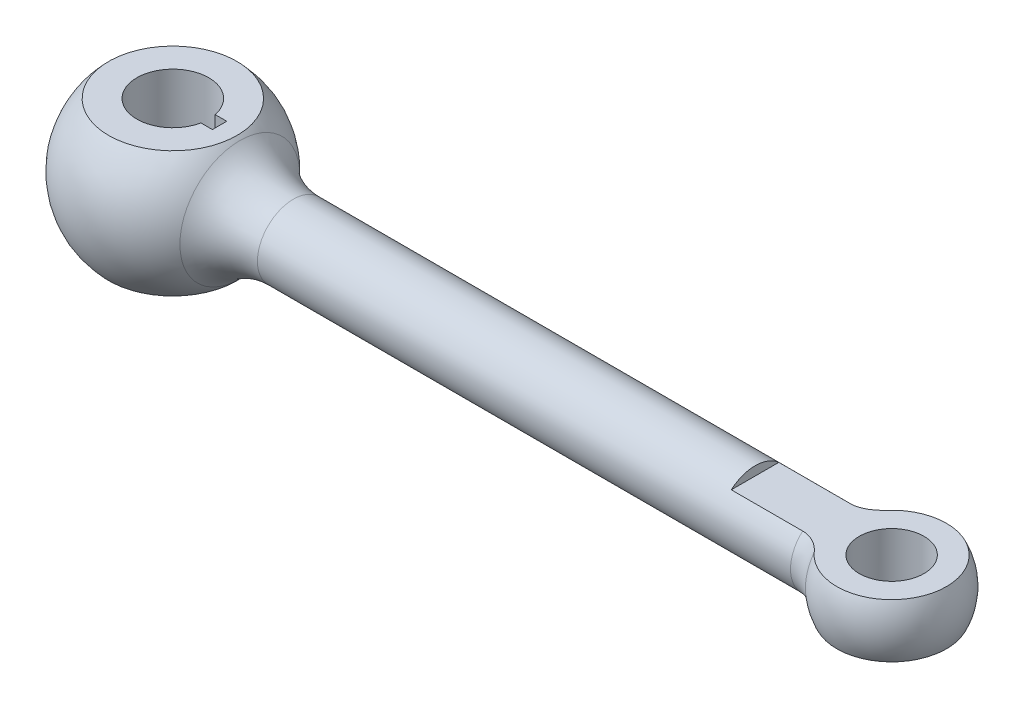
ISO-10303-21;
HEADER;
FILE_DESCRIPTION(('STEP AP214'),'2;1');
FILE_NAME('part.step','',(''),(''),'','','');
FILE_SCHEMA(('AUTOMOTIVE_DESIGN { 1 0 10303 214 1 1 1 1 }'));
ENDSEC;
DATA;
#1=APPLICATION_CONTEXT('core data for automotive mechanical design processes');
#2=APPLICATION_PROTOCOL_DEFINITION('international standard','automotive_design',2000,#1);
#3=PRODUCT_CONTEXT('',#1,'mechanical');
#4=PRODUCT('Part','Part','',(#3));
#5=PRODUCT_RELATED_PRODUCT_CATEGORY('part','',(#4));
#6=PRODUCT_DEFINITION_FORMATION('','',#4);
#7=PRODUCT_DEFINITION_CONTEXT('part definition',#1,'design');
#8=PRODUCT_DEFINITION('design','',#6,#7);
#9=PRODUCT_DEFINITION_SHAPE('','',#8);
#10=(LENGTH_UNIT() NAMED_UNIT(*) SI_UNIT(.MILLI.,.METRE.));
#11=(NAMED_UNIT(*) PLANE_ANGLE_UNIT() SI_UNIT($,.RADIAN.));
#12=(NAMED_UNIT(*) SI_UNIT($,.STERADIAN.) SOLID_ANGLE_UNIT());
#13=UNCERTAINTY_MEASURE_WITH_UNIT(LENGTH_MEASURE(1.E-05),#10,'distance_accuracy_value','');
#14=(GEOMETRIC_REPRESENTATION_CONTEXT(3) GLOBAL_UNCERTAINTY_ASSIGNED_CONTEXT((#13)) GLOBAL_UNIT_ASSIGNED_CONTEXT((#10,
#11,#12)) REPRESENTATION_CONTEXT('',''));
#15=CARTESIAN_POINT('',(0.,0.,0.));
#16=DIRECTION('',(0.,0.,1.));
#17=DIRECTION('',(1.,0.,0.));
#18=AXIS2_PLACEMENT_3D('',#15,#16,#17);
#19=CARTESIAN_POINT('',(-25.,0.,0.));
#20=DIRECTION('',(-1.,0.,0.));
#21=DIRECTION('',(0.,1.,0.));
#22=AXIS2_PLACEMENT_3D('',#19,#20,#21);
#23=SPHERICAL_SURFACE('',#22,25.);
#24=CARTESIAN_POINT('',(-6.36610018750175,0.,0.));
#25=DIRECTION('',(-1.,0.,0.));
#26=DIRECTION('',(0.,0.,1.));
#27=AXIS2_PLACEMENT_3D('',#24,#25,#26);
#28=CIRCLE('',#27,16.6666666666667);
#29=CARTESIAN_POINT('',(-6.36610018750175,0.,16.6666666666667));
#30=VERTEX_POINT('',#29);
#31=EDGE_CURVE('E198',#30,#30,#28,.T.);
#32=ORIENTED_EDGE('',*,*,#31,.T.);
#33=EDGE_LOOP('',(#32));
#34=FACE_BOUND('',#33,.T.);
#35=CARTESIAN_POINT('',(-25.,17.5,0.));
#36=DIRECTION('',(0.,1.,0.));
#37=DIRECTION('',(0.,0.,1.));
#38=AXIS2_PLACEMENT_3D('',#35,#36,#37);
#39=CIRCLE('',#38,17.8535710713571);
#40=CARTESIAN_POINT('',(-25.,17.5,17.8535710713571));
#41=VERTEX_POINT('',#40);
#42=EDGE_CURVE('E164',#41,#41,#39,.T.);
#43=ORIENTED_EDGE('',*,*,#42,.F.);
#44=EDGE_LOOP('',(#43));
#45=FACE_BOUND('',#44,.T.);
#46=CARTESIAN_POINT('',(-25.,-17.5,0.));
#47=DIRECTION('',(0.,-1.,0.));
#48=DIRECTION('',(0.,0.,-1.));
#49=AXIS2_PLACEMENT_3D('',#46,#47,#48);
#50=CIRCLE('',#49,17.8535710713571);
#51=CARTESIAN_POINT('',(-25.,-17.5,-17.8535710713571));
#52=VERTEX_POINT('',#51);
#53=EDGE_CURVE('E156',#52,#52,#50,.T.);
#54=ORIENTED_EDGE('',*,*,#53,.F.);
#55=EDGE_LOOP('',(#54));
#56=FACE_BOUND('',#55,.T.);
#57=CARTESIAN_POINT('',(-49.6779253585061,0.,0.));
#58=DIRECTION('',(1.,0.,0.));
#59=DIRECTION('',(0.,0.,-1.));
#60=AXIS2_PLACEMENT_3D('',#57,#58,#59);
#61=CIRCLE('',#60,4.);
#62=CARTESIAN_POINT('',(-49.6779253585061,0.,-4.));
#63=VERTEX_POINT('',#62);
#64=EDGE_CURVE('E293',#63,#63,#61,.F.);
#65=ORIENTED_EDGE('',*,*,#64,.F.);
#66=EDGE_LOOP('',(#65));
#67=FACE_BOUND('',#66,.T.);
#68=ADVANCED_FACE('F41',(#34,#45,#56,#67),#23,.T.);
#69=CARTESIAN_POINT('',(-25.,-22.5,0.));
#70=DIRECTION('',(0.,1.,0.));
#71=DIRECTION('',(0.,0.,1.));
#72=AXIS2_PLACEMENT_3D('',#69,#70,#71);
#73=CYLINDRICAL_SURFACE('',#72,10.);
#74=CARTESIAN_POINT('',(-25.,-17.5,0.));
#75=DIRECTION('',(0.,-1.,0.));
#76=DIRECTION('',(0.,0.,-1.));
#77=AXIS2_PLACEMENT_3D('',#74,#75,#76);
#78=CIRCLE('',#77,10.);
#79=CARTESIAN_POINT('',(-15.2020410288673,-17.5,2.));
#80=VERTEX_POINT('',#79);
#81=CARTESIAN_POINT('',(-15.2020410288673,-17.5,-2.));
#82=VERTEX_POINT('',#81);
#83=EDGE_CURVE('E133',#80,#82,#78,.T.);
#84=ORIENTED_EDGE('',*,*,#83,.T.);
#85=DIRECTION('',(0.,1.,0.));
#86=VECTOR('',#85,1.);
#87=CARTESIAN_POINT('',(-15.2020410288673,-22.5,-2.));
#88=LINE('',#87,#86);
#89=CARTESIAN_POINT('',(-15.2020410288673,17.5,-2.));
#90=VERTEX_POINT('',#89);
#91=EDGE_CURVE('E121',#82,#90,#88,.T.);
#92=ORIENTED_EDGE('',*,*,#91,.T.);
#93=CARTESIAN_POINT('',(-25.,17.5,0.));
#94=DIRECTION('',(0.,1.,0.));
#95=DIRECTION('',(0.,0.,1.));
#96=AXIS2_PLACEMENT_3D('',#93,#94,#95);
#97=CIRCLE('',#96,10.);
#98=CARTESIAN_POINT('',(-15.2020410288673,17.5,2.));
#99=VERTEX_POINT('',#98);
#100=EDGE_CURVE('E129',#90,#99,#97,.T.);
#101=ORIENTED_EDGE('',*,*,#100,.T.);
#102=DIRECTION('',(0.,1.,0.));
#103=VECTOR('',#102,1.);
#104=CARTESIAN_POINT('',(-15.2020410288673,-22.5,2.));
#105=LINE('',#104,#103);
#106=EDGE_CURVE('E138',#80,#99,#105,.T.);
#107=ORIENTED_EDGE('',*,*,#106,.F.);
#108=EDGE_LOOP('',(#84,#92,#101,#107));
#109=FACE_BOUND('',#108,.T.);
#110=CARTESIAN_POINT('',(-34.1651513899117,0.,4.));
#111=CARTESIAN_POINT('',(-34.1651522072251,-0.107177496784384,3.99999917996685));
#112=CARTESIAN_POINT('',(-34.1670378270459,-0.214387859794794,3.99568627578832));
#113=CARTESIAN_POINT('',(-34.1745189058127,-0.428032094170665,3.97847804504315));
#114=CARTESIAN_POINT('',(-34.1801166353845,-0.534465449945316,3.965577465543));
#115=CARTESIAN_POINT('',(-34.1948507861607,-0.745935953355521,3.9312935770878));
#116=CARTESIAN_POINT('',(-34.2039942584833,-0.850969884848686,3.90989336356571));
#117=CARTESIAN_POINT('',(-34.2255144619826,-1.05868759718977,3.85883937208579));
#118=CARTESIAN_POINT('',(-34.2378925354171,-1.16137038310176,3.82918216740128));
#119=CARTESIAN_POINT('',(-34.2792023148764,-1.46398972662859,3.72849978450445));
#120=CARTESIAN_POINT('',(-34.3123881019352,-1.65953792096433,3.64559228099563));
#121=CARTESIAN_POINT('',(-34.3862951267144,-2.03380126867295,3.45083256453889));
#122=CARTESIAN_POINT('',(-34.4270147185353,-2.21252008589124,3.33898667159604));
#123=CARTESIAN_POINT('',(-34.5140167746093,-2.55851181360141,3.08264624953204));
#124=CARTESIAN_POINT('',(-34.5604782179202,-2.72471043328898,2.93675933272146));
#125=CARTESIAN_POINT('',(-34.6522492808802,-3.03106040804192,2.61941759406606));
#126=CARTESIAN_POINT('',(-34.6975584932633,-3.17120266075496,2.44795387495429));
#127=CARTESIAN_POINT('',(-34.7840681180817,-3.42681210983709,2.07601279575004));
#128=CARTESIAN_POINT('',(-34.8250360629585,-3.54108841996941,1.87465797803874));
#129=CARTESIAN_POINT('',(-34.8960785633395,-3.73368731967694,1.45365059895514));
#130=CARTESIAN_POINT('',(-34.9261575504962,-3.81202453943324,1.23400552632834));
#131=CARTESIAN_POINT('',(-34.9707664974986,-3.92668292732297,0.793932865332428));
#132=CARTESIAN_POINT('',(-34.9859787347939,-3.96485461599806,0.574057972725524));
#133=CARTESIAN_POINT('',(-35.001606214367,-4.00405698350082,0.130532654160158));
#134=CARTESIAN_POINT('',(-35.0020269755724,-4.0051015150445,-0.0931163324631207));
#135=CARTESIAN_POINT('',(-34.9884392562601,-3.97103445745354,-0.524464988663932));
#136=CARTESIAN_POINT('',(-34.9752399353889,-3.93795045370289,-0.732354905542457));
#137=CARTESIAN_POINT('',(-34.9369858294236,-3.8400142481818,-1.1393462186423));
#138=CARTESIAN_POINT('',(-34.9119301744378,-3.77515971541564,-1.33844696883603));
#139=CARTESIAN_POINT('',(-34.8519364891382,-3.61472703402771,-1.72579587696675));
#140=CARTESIAN_POINT('',(-34.8168552093215,-3.51870057031128,-1.91383524674319));
#141=CARTESIAN_POINT('',(-34.7402917036085,-3.29906998621966,-2.27161630149723));
#142=CARTESIAN_POINT('',(-34.6988072853438,-3.17545641381566,-2.44135168543995));
#143=CARTESIAN_POINT('',(-34.6104327435216,-2.8947017280952,-2.76953765597606));
#144=CARTESIAN_POINT('',(-34.5633665302349,-2.73589221484983,-2.92651569053149));
#145=CARTESIAN_POINT('',(-34.4712332194655,-2.39401885634057,-3.21221483078645));
#146=CARTESIAN_POINT('',(-34.4261667801616,-2.21094710361003,-3.34092668757428));
#147=CARTESIAN_POINT('',(-34.3419379481804,-1.81916195525085,-3.56980837743822));
#148=CARTESIAN_POINT('',(-34.3029782811541,-1.60987033932236,-3.66906930327244));
#149=CARTESIAN_POINT('',(-34.2377518068817,-1.1755690193759,-3.83035251973301));
#150=CARTESIAN_POINT('',(-34.2114767578262,-0.950569630546911,-3.89239899675599));
#151=CARTESIAN_POINT('',(-34.1765951940543,-0.50592844506505,-3.97390989770977));
#152=CARTESIAN_POINT('',(-34.1670073291228,-0.286799105742873,-3.99574419362908));
#153=CARTESIAN_POINT('',(-34.1637899573808,0.152154415519103,-4.00312265288578));
#154=CARTESIAN_POINT('',(-34.1701556112072,0.371978366551337,-3.98867782118257));
#155=CARTESIAN_POINT('',(-34.1971208871823,0.792917869913856,-3.92606578958006));
#156=CARTESIAN_POINT('',(-34.216889155966,0.994385874799997,-3.87986612404771));
#157=CARTESIAN_POINT('',(-34.2674010205468,1.38657680957103,-3.75760837382175));
#158=CARTESIAN_POINT('',(-34.2981470497719,1.57729734621477,-3.68154366860459));
#159=CARTESIAN_POINT('',(-34.368675637202,1.95120471559083,-3.49827127896311));
#160=CARTESIAN_POINT('',(-34.4087740927836,2.13377237738722,-3.38992573652914));
#161=CARTESIAN_POINT('',(-34.4930077031559,2.47896597488502,-3.14633044888379));
#162=CARTESIAN_POINT('',(-34.5371444979208,2.64158374559781,-3.01106974696435));
#163=CARTESIAN_POINT('',(-34.6284183194284,2.95474681719132,-2.70568842336055));
#164=CARTESIAN_POINT('',(-34.6755361457051,3.10351313055453,-2.53373085888854));
#165=CARTESIAN_POINT('',(-34.7643958913502,3.3703541532482,-2.16616726673934));
#166=CARTESIAN_POINT('',(-34.8061375918612,3.48842761329747,-1.97056027694192));
#167=CARTESIAN_POINT('',(-34.8796743180093,3.69009525281948,-1.56055986799732));
#168=CARTESIAN_POINT('',(-34.9114717248188,3.77369768794723,-1.346170961965));
#169=CARTESIAN_POINT('',(-34.9614542693725,3.90309770519939,-0.904787181861568));
#170=CARTESIAN_POINT('',(-34.9796467941012,3.94891580431339,-0.677799220674799));
#171=CARTESIAN_POINT('',(-34.9995801642567,3.99900940191103,-0.233633020611975));
#172=CARTESIAN_POINT('',(-35.0023169350655,4.00580025207679,-0.0167809848943052));
#173=CARTESIAN_POINT('',(-34.9937208474038,3.98428904627956,0.414867671174724));
#174=CARTESIAN_POINT('',(-34.9823901187126,3.95599230247905,0.62966459770289));
#175=CARTESIAN_POINT('',(-34.9474302678916,3.86690640578721,1.04434180494581));
#176=CARTESIAN_POINT('',(-34.9241896149174,3.80714204349495,1.2444776131699));
#177=CARTESIAN_POINT('',(-34.8678989544096,3.65789445524216,1.63184470564404));
#178=CARTESIAN_POINT('',(-34.8348471377614,3.56840574794402,1.81907360209111));
#179=CARTESIAN_POINT('',(-34.7603618958876,3.3577933524316,2.18440609879393));
#180=CARTESIAN_POINT('',(-34.7186226276455,3.23544645590386,2.3617408310488));
#181=CARTESIAN_POINT('',(-34.6317880306343,2.96442391636386,2.69410799958837));
#182=CARTESIAN_POINT('',(-34.5866913172977,2.81573737596091,2.84913115669899));
#183=CARTESIAN_POINT('',(-34.4947554025592,2.48536576113423,3.14240275826141));
#184=CARTESIAN_POINT('',(-34.4479811565371,2.30220770129796,3.27901865020172));
#185=CARTESIAN_POINT('',(-34.3609929250149,1.91413027875233,3.51969402497221));
#186=CARTESIAN_POINT('',(-34.3207797110774,1.70920836133381,3.62374968011082));
#187=CARTESIAN_POINT('',(-34.2551790064237,1.30187605622044,3.78798515690828));
#188=CARTESIAN_POINT('',(-34.228784514946,1.10089232405414,3.85126569346865));
#189=CARTESIAN_POINT('',(-34.1988556584339,0.793361040209279,3.92194632104984));
#190=CARTESIAN_POINT('',(-34.1904927063377,0.68992696410562,3.94146052144918));
#191=CARTESIAN_POINT('',(-34.1772120034161,0.481643070389122,3.97228850679684));
#192=CARTESIAN_POINT('',(-34.1722922529317,0.376794110604086,3.98360705155155));
#193=CARTESIAN_POINT('',(-34.1678367542342,0.226449408647594,3.99384232103283));
#194=CARTESIAN_POINT('',(-34.1668305981541,0.181200169677813,3.99615058414993));
#195=CARTESIAN_POINT('',(-34.1654877186478,0.0906359157853919,3.99922965337524));
#196=CARTESIAN_POINT('',(-34.1651510443039,0.0453208962838169,4.00000034675784));
#197=CARTESIAN_POINT('',(-34.1651513899117,0.,4.));
#198=B_SPLINE_CURVE_WITH_KNOTS('',3,(#110,#111,#112,#113,#114,#115,#116,#117,#118,#119,#120,
#121,#122,#123,#124,#125,#126,#127,#128,#129,#130,#131,#132,#133,#134,#135,#136,#137,#138,#139,
#140,#141,#142,#143,#144,#145,#146,#147,#148,#149,#150,#151,#152,#153,#154,#155,#156,#157,#158,
#159,#160,#161,#162,#163,#164,#165,#166,#167,#168,#169,#170,#171,#172,#173,#174,#175,#176,#177,
#178,#179,#180,#181,#182,#183,#184,#185,#186,#187,#188,#189,#190,#191,#192,#193,#194,#195,#196,
#197),.UNSPECIFIED.,.T.,.F.,(4,2,2,2,2,2,2,2,2,2,2,2,2,2,2,2,2,2,2,2,2,2,2,2,2,2,2,2,2,2,2,2,2,
2,2,2,2,2,2,2,2,2,2,4),(0.,0.321486083338404,0.64316899511119,0.965494918272705,
1.28795480954363,1.92974178448592,2.57138871437637,3.24631250358764,3.92147162486599,
4.62325351972771,5.32474947728875,5.99228379564281,6.65956904401258,7.28937303450519,
7.91922324048033,8.5585661425971,9.19812843669976,9.87968101952625,10.5614562804417,
11.2624893122443,11.9630662339012,12.6208430883876,13.2784204360579,13.898545099602,
14.5188073109319,15.1642232309532,15.8099024284161,16.5032748228387,17.1966754349541,
17.8899098841554,18.5827676569819,19.2304209330182,19.8779761681512,20.5056400267662,
21.1334196944708,21.7889411606976,22.4447344691833,23.1411252036114,23.8375977730829,
24.4715333542807,24.7879924179096,25.1042675432749,25.240200643082,25.3761437083411),.UNSPECIFIED.);
#199=CARTESIAN_POINT('',(-34.1651513899117,0.,4.));
#200=VERTEX_POINT('',#199);
#201=EDGE_CURVE('E46',#200,#200,#198,.T.);
#202=ORIENTED_EDGE('',*,*,#201,.F.);
#203=EDGE_LOOP('',(#202));
#204=FACE_BOUND('',#203,.T.);
#205=ADVANCED_FACE('F126',(#109,#204),#73,.F.);
#206=CARTESIAN_POINT('',(175.,0.,0.));
#207=DIRECTION('',(-1.,0.,0.));
#208=DIRECTION('',(0.,1.,0.));
#209=AXIS2_PLACEMENT_3D('',#206,#207,#208);
#210=SPHERICAL_SURFACE('',#209,17.);
#211=CARTESIAN_POINT('',(175.,-7.5,0.));
#212=DIRECTION('',(0.,-1.,0.));
#213=DIRECTION('',(0.,0.,-1.));
#214=AXIS2_PLACEMENT_3D('',#211,#212,#213);
#215=CIRCLE('',#214,15.2561463023924);
#216=CARTESIAN_POINT('',(163.579552907308,-7.5,-10.1155023702739));
#217=VERTEX_POINT('',#216);
#218=CARTESIAN_POINT('',(163.579552907308,-7.5,10.1155023702739));
#219=VERTEX_POINT('',#218);
#220=EDGE_CURVE('E165',#217,#219,#215,.T.);
#221=ORIENTED_EDGE('',*,*,#220,.F.);
#222=CARTESIAN_POINT('',(163.579552907308,0.,0.));
#223=DIRECTION('',(1.,0.,0.));
#224=DIRECTION('',(0.,0.,-1.));
#225=AXIS2_PLACEMENT_3D('',#222,#223,#224);
#226=CIRCLE('',#225,12.5925925925926);
#227=CARTESIAN_POINT('',(163.579552907308,7.5,-10.1155023702739));
#228=VERTEX_POINT('',#227);
#229=EDGE_CURVE('E62',#217,#228,#226,.T.);
#230=ORIENTED_EDGE('',*,*,#229,.T.);
#231=CARTESIAN_POINT('',(175.,7.5,0.));
#232=DIRECTION('',(0.,1.,0.));
#233=DIRECTION('',(0.,0.,1.));
#234=AXIS2_PLACEMENT_3D('',#231,#232,#233);
#235=CIRCLE('',#234,15.2561463023924);
#236=CARTESIAN_POINT('',(163.579552907308,7.5,10.1155023702739));
#237=VERTEX_POINT('',#236);
#238=EDGE_CURVE('E167',#237,#228,#235,.T.);
#239=ORIENTED_EDGE('',*,*,#238,.F.);
#240=CARTESIAN_POINT('',(163.579552907308,0.,0.));
#241=DIRECTION('',(1.,0.,0.));
#242=DIRECTION('',(0.,0.,-1.));
#243=AXIS2_PLACEMENT_3D('',#240,#241,#242);
#244=CIRCLE('',#243,12.5925925925926);
#245=EDGE_CURVE('E213',#237,#219,#244,.T.);
#246=ORIENTED_EDGE('',*,*,#245,.T.);
#247=EDGE_LOOP('',(#221,#230,#239,#246));
#248=FACE_BOUND('',#247,.T.);
#249=ADVANCED_FACE('F262',(#248),#210,.T.);
#250=CARTESIAN_POINT('',(0.,0.,0.));
#251=DIRECTION('',(-1.,0.,0.));
#252=DIRECTION('',(0.,0.,1.));
#253=AXIS2_PLACEMENT_3D('',#250,#251,#252);
#254=CYLINDRICAL_SURFACE('',#253,10.);
#255=CARTESIAN_POINT('',(8.54101966249685,0.,0.));
#256=DIRECTION('',(-1.,0.,0.));
#257=DIRECTION('',(0.,0.,1.));
#258=AXIS2_PLACEMENT_3D('',#255,#256,#257);
#259=CIRCLE('',#258,10.);
#260=CARTESIAN_POINT('',(8.54101966249685,0.,10.));
#261=VERTEX_POINT('',#260);
#262=EDGE_CURVE('E202',#261,#261,#259,.F.);
#263=ORIENTED_EDGE('',*,*,#262,.T.);
#264=EDGE_LOOP('',(#263));
#265=FACE_BOUND('',#264,.T.);
#266=DIRECTION('',(-1.,0.,0.));
#267=VECTOR('',#266,1.);
#268=CARTESIAN_POINT('',(0.,7.5,-6.61437827766147));
#269=LINE('',#268,#267);
#270=CARTESIAN_POINT('',(156.861642852783,7.5,-6.61437827766147));
#271=VERTEX_POINT('',#270);
#272=CARTESIAN_POINT('',(137.002179540985,7.5,-6.61437827766147));
#273=VERTEX_POINT('',#272);
#274=EDGE_CURVE('E180',#271,#273,#269,.T.);
#275=ORIENTED_EDGE('',*,*,#274,.F.);
#276=CARTESIAN_POINT('',(156.861642852783,0.,0.));
#277=DIRECTION('',(1.,0.,0.));
#278=DIRECTION('',(0.,0.,-1.));
#279=AXIS2_PLACEMENT_3D('',#276,#277,#278);
#280=CIRCLE('',#279,10.);
#281=CARTESIAN_POINT('',(156.861642852783,-7.5,-6.61437827766147));
#282=VERTEX_POINT('',#281);
#283=EDGE_CURVE('E211',#271,#282,#280,.F.);
#284=ORIENTED_EDGE('',*,*,#283,.T.);
#285=DIRECTION('',(-1.,0.,0.));
#286=VECTOR('',#285,1.);
#287=CARTESIAN_POINT('',(0.,-7.5,-6.61437827766147));
#288=LINE('',#287,#286);
#289=CARTESIAN_POINT('',(137.002179540985,-7.5,-6.61437827766147));
#290=VERTEX_POINT('',#289);
#291=EDGE_CURVE('E177',#290,#282,#288,.F.);
#292=ORIENTED_EDGE('',*,*,#291,.F.);
#293=CARTESIAN_POINT('',(137.002179540985,0.,0.));
#294=DIRECTION('',(-1.,0.,0.));
#295=DIRECTION('',(0.,0.,1.));
#296=AXIS2_PLACEMENT_3D('',#293,#294,#295);
#297=CIRCLE('',#296,10.);
#298=CARTESIAN_POINT('',(137.002179540985,-7.5,6.61437827766147));
#299=VERTEX_POINT('',#298);
#300=EDGE_CURVE('E185',#290,#299,#297,.T.);
#301=ORIENTED_EDGE('',*,*,#300,.T.);
#302=DIRECTION('',(-1.,0.,0.));
#303=VECTOR('',#302,1.);
#304=CARTESIAN_POINT('',(0.,-7.5,6.61437827766147));
#305=LINE('',#304,#303);
#306=CARTESIAN_POINT('',(156.861642852783,-7.5,6.61437827766147));
#307=VERTEX_POINT('',#306);
#308=EDGE_CURVE('E184',#307,#299,#305,.T.);
#309=ORIENTED_EDGE('',*,*,#308,.F.);
#310=CARTESIAN_POINT('',(156.861642852783,0.,0.));
#311=DIRECTION('',(1.,0.,0.));
#312=DIRECTION('',(0.,0.,-1.));
#313=AXIS2_PLACEMENT_3D('',#310,#311,#312);
#314=CIRCLE('',#313,10.);
#315=CARTESIAN_POINT('',(156.861642852783,7.5,6.61437827766147));
#316=VERTEX_POINT('',#315);
#317=EDGE_CURVE('E206',#307,#316,#314,.F.);
#318=ORIENTED_EDGE('',*,*,#317,.T.);
#319=DIRECTION('',(-1.,0.,0.));
#320=VECTOR('',#319,1.);
#321=CARTESIAN_POINT('',(0.,7.5,6.61437827766147));
#322=LINE('',#321,#320);
#323=CARTESIAN_POINT('',(137.002179540985,7.5,6.61437827766147));
#324=VERTEX_POINT('',#323);
#325=EDGE_CURVE('E175',#324,#316,#322,.F.);
#326=ORIENTED_EDGE('',*,*,#325,.F.);
#327=CARTESIAN_POINT('',(137.002179540985,0.,0.));
#328=DIRECTION('',(1.,0.,0.));
#329=DIRECTION('',(0.,0.,-1.));
#330=AXIS2_PLACEMENT_3D('',#327,#328,#329);
#331=CIRCLE('',#330,10.);
#332=EDGE_CURVE('E172',#273,#324,#331,.T.);
#333=ORIENTED_EDGE('',*,*,#332,.F.);
#334=EDGE_LOOP('',(#275,#284,#292,#301,#309,#318,#326,#333));
#335=FACE_BOUND('',#334,.T.);
#336=ADVANCED_FACE('F259',(#265,#335),#254,.T.);
#337=CARTESIAN_POINT('',(137.002179540985,17.5,-20.2694187702266));
#338=DIRECTION('',(1.,0.,0.));
#339=DIRECTION('',(0.,0.,-1.));
#340=AXIS2_PLACEMENT_3D('',#337,#338,#339);
#341=PLANE('',#340);
#342=ORIENTED_EDGE('',*,*,#332,.T.);
#343=DIRECTION('',(0.,0.,1.));
#344=VECTOR('',#343,1.);
#345=CARTESIAN_POINT('',(137.002179540985,7.5,-20.2694187702266));
#346=LINE('',#345,#344);
#347=EDGE_CURVE('E166',#273,#324,#346,.T.);
#348=ORIENTED_EDGE('',*,*,#347,.F.);
#349=EDGE_LOOP('',(#342,#348));
#350=FACE_BOUND('',#349,.T.);
#351=ADVANCED_FACE('F253',(#350),#341,.T.);
#352=CARTESIAN_POINT('',(0.,7.5,0.));
#353=DIRECTION('',(0.,1.,0.));
#354=DIRECTION('',(0.,0.,1.));
#355=AXIS2_PLACEMENT_3D('',#352,#353,#354);
#356=PLANE('',#355);
#357=CARTESIAN_POINT('',(175.,7.5,0.));
#358=DIRECTION('',(0.,1.,0.));
#359=DIRECTION('',(0.,0.,1.));
#360=AXIS2_PLACEMENT_3D('',#357,#358,#359);
#361=CIRCLE('',#360,9.00000000000001);
#362=CARTESIAN_POINT('',(175.,7.5,9.00000000000001));
#363=VERTEX_POINT('',#362);
#364=EDGE_CURVE('E205',#363,#363,#361,.T.);
#365=ORIENTED_EDGE('',*,*,#364,.F.);
#366=EDGE_LOOP('',(#365));
#367=FACE_BOUND('',#366,.T.);
#368=ORIENTED_EDGE('',*,*,#238,.T.);
#369=CARTESIAN_POINT('',(163.579552907308,7.5,-10.1155023702739));
#370=CARTESIAN_POINT('',(163.474769834163,7.5,-9.99720726138382));
#371=CARTESIAN_POINT('',(163.3678618628,7.5,-9.88080970811956));
#372=CARTESIAN_POINT('',(163.149837656753,7.5,-9.65200955610534));
#373=CARTESIAN_POINT('',(163.038721113773,7.5,-9.53960725119778));
#374=CARTESIAN_POINT('',(162.698727604228,7.5,-9.20831245884123));
#375=CARTESIAN_POINT('',(162.463593029927,7.5,-8.99576936234443));
#376=CARTESIAN_POINT('',(161.973130319847,7.5,-8.58661619341136));
#377=CARTESIAN_POINT('',(161.717532005201,7.5,-8.39032873131534));
#378=CARTESIAN_POINT('',(161.190347543977,7.5,-8.02110441295629));
#379=CARTESIAN_POINT('',(160.918775780457,7.5,-7.84814699808274));
#380=CARTESIAN_POINT('',(160.26295451581,7.5,-7.47440052714146));
#381=CARTESIAN_POINT('',(159.872185695544,7.5,-7.28463335372538));
#382=CARTESIAN_POINT('',(159.269067190411,7.5,-7.04814733941781));
#383=CARTESIAN_POINT('',(159.065931678387,7.5,-6.97750828643357));
#384=CARTESIAN_POINT('',(158.65444068621,7.5,-6.85369940596053));
#385=CARTESIAN_POINT('',(158.446087612678,7.5,-6.80052167847359));
#386=CARTESIAN_POINT('',(158.01048008529,7.5,-6.71025341266789));
#387=CARTESIAN_POINT('',(157.782929072302,7.5,-6.67456227561141));
#388=CARTESIAN_POINT('',(157.439215061707,7.5,-6.63858866966147));
#389=CARTESIAN_POINT('',(157.323917836321,7.5,-6.62952413667485));
#390=CARTESIAN_POINT('',(157.092968815727,7.5,-6.61741406589461));
#391=CARTESIAN_POINT('',(156.977316912966,7.5,-6.61437058275184));
#392=CARTESIAN_POINT('',(156.861642852783,7.5,-6.61437827766147));
#393=B_SPLINE_CURVE_WITH_KNOTS('',3,(#369,#370,#371,#372,#373,#374,#375,#376,#377,#378,#379,
#380,#381,#382,#383,#384,#385,#386,#387,#388,#389,#390,#391,#392),.UNSPECIFIED.,.F.,.F.,(4,2,2,
2,2,2,2,2,2,2,2,4),(0.,0.474036656551859,0.948108105696828,1.89799697678677,2.86363556209121,
3.82841758163828,5.12644490386445,5.77101491101689,6.41529289334001,7.10501836282089,
7.45183935202879,7.79877867163184),.UNSPECIFIED.);
#394=EDGE_CURVE('E224',#228,#271,#393,.T.);
#395=ORIENTED_EDGE('',*,*,#394,.T.);
#396=ORIENTED_EDGE('',*,*,#274,.T.);
#397=ORIENTED_EDGE('',*,*,#347,.T.);
#398=ORIENTED_EDGE('',*,*,#325,.T.);
#399=CARTESIAN_POINT('',(156.861642852783,7.5,6.61437827766147));
#400=CARTESIAN_POINT('',(156.978718981189,7.5,6.61436537547752));
#401=CARTESIAN_POINT('',(157.095790003373,7.5,6.61748635841604));
#402=CARTESIAN_POINT('',(157.329586048896,7.5,6.62989960137549));
#403=CARTESIAN_POINT('',(157.446311125305,7.5,6.63919085972964));
#404=CARTESIAN_POINT('',(157.678890680255,7.5,6.66382417376256));
#405=CARTESIAN_POINT('',(157.794746412737,7.5,6.67915439326618));
#406=CARTESIAN_POINT('',(158.025521155016,7.5,6.71568182750459));
#407=CARTESIAN_POINT('',(158.140440137299,7.5,6.73687921394221));
#408=CARTESIAN_POINT('',(158.480369960769,7.5,6.80831037403592));
#409=CARTESIAN_POINT('',(158.703705459786,7.5,6.86672863148083));
#410=CARTESIAN_POINT('',(159.144207461786,7.5,7.0034637798633));
#411=CARTESIAN_POINT('',(159.361371112734,7.5,7.08178970917642));
#412=CARTESIAN_POINT('',(159.786670880194,7.5,7.25530329193259));
#413=CARTESIAN_POINT('',(159.994867796626,7.5,7.35034279209469));
#414=CARTESIAN_POINT('',(160.403562374738,7.5,7.55562714513321));
#415=CARTESIAN_POINT('',(160.604060514978,7.5,7.66587105093353));
#416=CARTESIAN_POINT('',(160.998074881118,7.5,7.90036091770959));
#417=CARTESIAN_POINT('',(161.191549310851,7.5,8.02467680582048));
#418=CARTESIAN_POINT('',(161.570233804941,7.5,8.28531892470298));
#419=CARTESIAN_POINT('',(161.75544317311,7.5,8.4216461643554));
#420=CARTESIAN_POINT('',(162.085608824903,7.5,8.68013427269151));
#421=CARTESIAN_POINT('',(162.231919209356,7.5,8.8005745126537));
#422=CARTESIAN_POINT('',(162.518724288325,7.5,9.04817416826897));
#423=CARTESIAN_POINT('',(162.659219307179,7.5,9.17533320829355));
#424=CARTESIAN_POINT('',(162.933109814946,7.5,9.43474456139496));
#425=CARTESIAN_POINT('',(163.066556374469,7.5,9.56694303436916));
#426=CARTESIAN_POINT('',(163.327523242921,7.5,9.83704319963487));
#427=CARTESIAN_POINT('',(163.455044110112,7.5,9.97494435235086));
#428=CARTESIAN_POINT('',(163.579552907308,7.5,10.1155023702739));
#429=B_SPLINE_CURVE_WITH_KNOTS('',3,(#399,#400,#401,#402,#403,#404,#405,#406,#407,#408,#409,
#410,#411,#412,#413,#414,#415,#416,#417,#418,#419,#420,#421,#422,#423,#424,#425,#426,#427,#428),
.UNSPECIFIED.,.F.,.F.,(4,2,2,2,2,2,2,2,2,2,2,2,2,2,4),(0.,0.351178227622914,0.70229945979881,
1.05273590229769,1.40318260141477,2.09460649299127,2.78634486367997,3.4722350384791,
4.1580825087439,4.84750158484224,5.53697862327434,6.10529061090185,6.67357085941402,
7.23691454193782,7.80020504348642),.UNSPECIFIED.);
#430=EDGE_CURVE('E57',#316,#237,#429,.T.);
#431=ORIENTED_EDGE('',*,*,#430,.T.);
#432=EDGE_LOOP('',(#368,#395,#396,#397,#398,#431));
#433=FACE_BOUND('',#432,.T.);
#434=ADVANCED_FACE('F252',(#367,#433),#356,.T.);
#435=CARTESIAN_POINT('',(137.002179540985,-17.5,-20.2694187702266));
#436=DIRECTION('',(-1.,0.,0.));
#437=DIRECTION('',(0.,0.,1.));
#438=AXIS2_PLACEMENT_3D('',#435,#436,#437);
#439=PLANE('',#438);
#440=DIRECTION('',(0.,0.,1.));
#441=VECTOR('',#440,1.);
#442=CARTESIAN_POINT('',(137.002179540985,-7.5,-20.2694187702266));
#443=LINE('',#442,#441);
#444=EDGE_CURVE('E163',#290,#299,#443,.T.);
#445=ORIENTED_EDGE('',*,*,#444,.T.);
#446=ORIENTED_EDGE('',*,*,#300,.F.);
#447=EDGE_LOOP('',(#445,#446));
#448=FACE_BOUND('',#447,.T.);
#449=ADVANCED_FACE('F237',(#448),#439,.F.);
#450=CARTESIAN_POINT('',(0.,-7.5,0.));
#451=DIRECTION('',(0.,-1.,0.));
#452=DIRECTION('',(0.,0.,1.));
#453=AXIS2_PLACEMENT_3D('',#450,#451,#452);
#454=PLANE('',#453);
#455=CARTESIAN_POINT('',(175.,-7.5,0.));
#456=DIRECTION('',(0.,-1.,0.));
#457=DIRECTION('',(0.,0.,-1.));
#458=AXIS2_PLACEMENT_3D('',#455,#456,#457);
#459=CIRCLE('',#458,9.00000000000001);
#460=CARTESIAN_POINT('',(175.,-7.5,-9.00000000000001));
#461=VERTEX_POINT('',#460);
#462=EDGE_CURVE('E197',#461,#461,#459,.T.);
#463=ORIENTED_EDGE('',*,*,#462,.F.);
#464=EDGE_LOOP('',(#463));
#465=FACE_BOUND('',#464,.T.);
#466=ORIENTED_EDGE('',*,*,#220,.T.);
#467=CARTESIAN_POINT('',(163.579552907308,-7.5,10.1155023702739));
#468=CARTESIAN_POINT('',(163.474769834163,-7.5,9.99720726138382));
#469=CARTESIAN_POINT('',(163.3678618628,-7.5,9.88080970811956));
#470=CARTESIAN_POINT('',(163.149837656753,-7.5,9.65200955610534));
#471=CARTESIAN_POINT('',(163.038721113773,-7.5,9.53960725119778));
#472=CARTESIAN_POINT('',(162.698727604228,-7.5,9.20831245884123));
#473=CARTESIAN_POINT('',(162.463593029927,-7.5,8.99576936234443));
#474=CARTESIAN_POINT('',(161.973130319847,-7.5,8.58661619341136));
#475=CARTESIAN_POINT('',(161.717532005201,-7.5,8.39032873131534));
#476=CARTESIAN_POINT('',(161.190347543977,-7.5,8.02110441295629));
#477=CARTESIAN_POINT('',(160.918775780457,-7.5,7.84814699808274));
#478=CARTESIAN_POINT('',(160.26295451581,-7.5,7.47440052714146));
#479=CARTESIAN_POINT('',(159.872185695544,-7.5,7.28463335372538));
#480=CARTESIAN_POINT('',(159.269067190411,-7.5,7.04814733941781));
#481=CARTESIAN_POINT('',(159.065931678387,-7.5,6.97750828643357));
#482=CARTESIAN_POINT('',(158.65444068621,-7.5,6.85369940596053));
#483=CARTESIAN_POINT('',(158.446087612678,-7.5,6.80052167847359));
#484=CARTESIAN_POINT('',(158.01048008529,-7.5,6.71025341266789));
#485=CARTESIAN_POINT('',(157.782929072302,-7.5,6.67456227561141));
#486=CARTESIAN_POINT('',(157.439215061707,-7.5,6.63858866966147));
#487=CARTESIAN_POINT('',(157.323917836321,-7.5,6.62952413667485));
#488=CARTESIAN_POINT('',(157.092968815727,-7.5,6.61741406589461));
#489=CARTESIAN_POINT('',(156.977316912966,-7.5,6.61437058275184));
#490=CARTESIAN_POINT('',(156.861642852783,-7.5,6.61437827766147));
#491=B_SPLINE_CURVE_WITH_KNOTS('',3,(#467,#468,#469,#470,#471,#472,#473,#474,#475,#476,#477,
#478,#479,#480,#481,#482,#483,#484,#485,#486,#487,#488,#489,#490),.UNSPECIFIED.,.F.,.F.,(4,2,2,
2,2,2,2,2,2,2,2,4),(0.,0.474036656551859,0.948108105696828,1.89799697678677,2.86363556209121,
3.82841758163828,5.12644490386445,5.77101491101689,6.41529289334001,7.10501836282089,
7.45183935202879,7.79877867163184),.UNSPECIFIED.);
#492=EDGE_CURVE('E11',#219,#307,#491,.T.);
#493=ORIENTED_EDGE('',*,*,#492,.T.);
#494=ORIENTED_EDGE('',*,*,#308,.T.);
#495=ORIENTED_EDGE('',*,*,#444,.F.);
#496=ORIENTED_EDGE('',*,*,#291,.T.);
#497=CARTESIAN_POINT('',(156.861642852783,-7.5,-6.61437827766147));
#498=CARTESIAN_POINT('',(156.978718981189,-7.5,-6.61436537547752));
#499=CARTESIAN_POINT('',(157.095790003373,-7.5,-6.61748635841604));
#500=CARTESIAN_POINT('',(157.329586048896,-7.5,-6.62989960137549));
#501=CARTESIAN_POINT('',(157.446311125305,-7.5,-6.63919085972964));
#502=CARTESIAN_POINT('',(157.678890680255,-7.5,-6.66382417376256));
#503=CARTESIAN_POINT('',(157.794746412737,-7.5,-6.67915439326618));
#504=CARTESIAN_POINT('',(158.025521155016,-7.5,-6.71568182750459));
#505=CARTESIAN_POINT('',(158.140440137299,-7.5,-6.73687921394221));
#506=CARTESIAN_POINT('',(158.480369960769,-7.5,-6.80831037403592));
#507=CARTESIAN_POINT('',(158.703705459786,-7.5,-6.86672863148083));
#508=CARTESIAN_POINT('',(159.144207461786,-7.5,-7.0034637798633));
#509=CARTESIAN_POINT('',(159.361371112734,-7.5,-7.08178970917642));
#510=CARTESIAN_POINT('',(159.786670880194,-7.5,-7.25530329193259));
#511=CARTESIAN_POINT('',(159.994867796626,-7.5,-7.35034279209469));
#512=CARTESIAN_POINT('',(160.403562374738,-7.5,-7.55562714513321));
#513=CARTESIAN_POINT('',(160.604060514978,-7.5,-7.66587105093353));
#514=CARTESIAN_POINT('',(160.998074881118,-7.5,-7.90036091770959));
#515=CARTESIAN_POINT('',(161.191549310851,-7.5,-8.02467680582048));
#516=CARTESIAN_POINT('',(161.570233804941,-7.5,-8.28531892470298));
#517=CARTESIAN_POINT('',(161.75544317311,-7.5,-8.4216461643554));
#518=CARTESIAN_POINT('',(162.085608824903,-7.5,-8.68013427269151));
#519=CARTESIAN_POINT('',(162.231919209356,-7.5,-8.8005745126537));
#520=CARTESIAN_POINT('',(162.518724288325,-7.5,-9.04817416826897));
#521=CARTESIAN_POINT('',(162.659219307179,-7.5,-9.17533320829355));
#522=CARTESIAN_POINT('',(162.933109814946,-7.5,-9.43474456139496));
#523=CARTESIAN_POINT('',(163.066556374469,-7.5,-9.56694303436916));
#524=CARTESIAN_POINT('',(163.327523242921,-7.5,-9.83704319963487));
#525=CARTESIAN_POINT('',(163.455044110112,-7.5,-9.97494435235086));
#526=CARTESIAN_POINT('',(163.579552907308,-7.5,-10.1155023702739));
#527=B_SPLINE_CURVE_WITH_KNOTS('',3,(#497,#498,#499,#500,#501,#502,#503,#504,#505,#506,#507,
#508,#509,#510,#511,#512,#513,#514,#515,#516,#517,#518,#519,#520,#521,#522,#523,#524,#525,#526),
.UNSPECIFIED.,.F.,.F.,(4,2,2,2,2,2,2,2,2,2,2,2,2,2,4),(0.,0.351178227622914,0.70229945979881,
1.05273590229769,1.40318260141477,2.09460649299127,2.78634486367997,3.4722350384791,
4.1580825087439,4.84750158484224,5.53697862327434,6.10529061090185,6.67357085941402,
7.23691454193782,7.80020504348642),.UNSPECIFIED.);
#528=EDGE_CURVE('E220',#282,#217,#527,.T.);
#529=ORIENTED_EDGE('',*,*,#528,.T.);
#530=EDGE_LOOP('',(#466,#493,#494,#495,#496,#529));
#531=FACE_BOUND('',#530,.T.);
#532=ADVANCED_FACE('F234',(#465,#531),#454,.T.);
#533=CARTESIAN_POINT('',(0.,17.5,0.));
#534=DIRECTION('',(0.,1.,0.));
#535=DIRECTION('',(0.,0.,1.));
#536=AXIS2_PLACEMENT_3D('',#533,#534,#535);
#537=PLANE('',#536);
#538=DIRECTION('',(0.,0.,-1.));
#539=VECTOR('',#538,1.);
#540=CARTESIAN_POINT('',(-12.,17.5,-2.));
#541=LINE('',#540,#539);
#542=CARTESIAN_POINT('',(-12.,17.5,2.));
#543=VERTEX_POINT('',#542);
#544=CARTESIAN_POINT('',(-12.,17.5,-2.));
#545=VERTEX_POINT('',#544);
#546=EDGE_CURVE('E146',#543,#545,#541,.T.);
#547=ORIENTED_EDGE('',*,*,#546,.F.);
#548=DIRECTION('',(1.,0.,0.));
#549=VECTOR('',#548,1.);
#550=CARTESIAN_POINT('',(-15.2020410288673,17.5,2.));
#551=LINE('',#550,#549);
#552=EDGE_CURVE('E151',#99,#543,#551,.T.);
#553=ORIENTED_EDGE('',*,*,#552,.F.);
#554=ORIENTED_EDGE('',*,*,#100,.F.);
#555=DIRECTION('',(-1.,0.,0.));
#556=VECTOR('',#555,1.);
#557=CARTESIAN_POINT('',(-15.2020410288673,17.5,-2.));
#558=LINE('',#557,#556);
#559=EDGE_CURVE('E142',#545,#90,#558,.T.);
#560=ORIENTED_EDGE('',*,*,#559,.F.);
#561=EDGE_LOOP('',(#547,#553,#554,#560));
#562=FACE_BOUND('',#561,.T.);
#563=ORIENTED_EDGE('',*,*,#42,.T.);
#564=EDGE_LOOP('',(#563));
#565=FACE_BOUND('',#564,.T.);
#566=ADVANCED_FACE('F147',(#562,#565),#537,.T.);
#567=CARTESIAN_POINT('',(0.,-17.5,0.));
#568=DIRECTION('',(0.,-1.,0.));
#569=DIRECTION('',(0.,0.,1.));
#570=AXIS2_PLACEMENT_3D('',#567,#568,#569);
#571=PLANE('',#570);
#572=DIRECTION('',(0.,0.,1.));
#573=VECTOR('',#572,1.);
#574=CARTESIAN_POINT('',(-12.,-17.5,0.));
#575=LINE('',#574,#573);
#576=CARTESIAN_POINT('',(-12.,-17.5,-2.));
#577=VERTEX_POINT('',#576);
#578=CARTESIAN_POINT('',(-12.,-17.5,2.));
#579=VERTEX_POINT('',#578);
#580=EDGE_CURVE('E196',#577,#579,#575,.T.);
#581=ORIENTED_EDGE('',*,*,#580,.F.);
#582=DIRECTION('',(1.,0.,0.));
#583=VECTOR('',#582,1.);
#584=CARTESIAN_POINT('',(0.,-17.5,-2.));
#585=LINE('',#584,#583);
#586=EDGE_CURVE('E190',#82,#577,#585,.T.);
#587=ORIENTED_EDGE('',*,*,#586,.F.);
#588=ORIENTED_EDGE('',*,*,#83,.F.);
#589=DIRECTION('',(-1.,0.,0.));
#590=VECTOR('',#589,1.);
#591=CARTESIAN_POINT('',(0.,-17.5,2.));
#592=LINE('',#591,#590);
#593=EDGE_CURVE('E193',#579,#80,#592,.T.);
#594=ORIENTED_EDGE('',*,*,#593,.F.);
#595=EDGE_LOOP('',(#581,#587,#588,#594));
#596=FACE_BOUND('',#595,.T.);
#597=ORIENTED_EDGE('',*,*,#53,.T.);
#598=EDGE_LOOP('',(#597));
#599=FACE_BOUND('',#598,.T.);
#600=ADVANCED_FACE('F304',(#596,#599),#571,.T.);
#601=CARTESIAN_POINT('',(-12.,-22.5,-2.));
#602=DIRECTION('',(1.,0.,0.));
#603=DIRECTION('',(0.,0.,-1.));
#604=AXIS2_PLACEMENT_3D('',#601,#602,#603);
#605=PLANE('',#604);
#606=ORIENTED_EDGE('',*,*,#580,.T.);
#607=DIRECTION('',(0.,1.,0.));
#608=VECTOR('',#607,1.);
#609=CARTESIAN_POINT('',(-12.,-22.5,2.));
#610=LINE('',#609,#608);
#611=EDGE_CURVE('E158',#579,#543,#610,.T.);
#612=ORIENTED_EDGE('',*,*,#611,.T.);
#613=ORIENTED_EDGE('',*,*,#546,.T.);
#614=DIRECTION('',(0.,1.,0.));
#615=VECTOR('',#614,1.);
#616=CARTESIAN_POINT('',(-12.,-22.5,-2.));
#617=LINE('',#616,#615);
#618=EDGE_CURVE('E140',#577,#545,#617,.T.);
#619=ORIENTED_EDGE('',*,*,#618,.F.);
#620=EDGE_LOOP('',(#606,#612,#613,#619));
#621=FACE_BOUND('',#620,.T.);
#622=ADVANCED_FACE('F296',(#621),#605,.F.);
#623=CARTESIAN_POINT('',(-15.2020410288673,-22.5,2.));
#624=DIRECTION('',(0.,0.,1.));
#625=DIRECTION('',(1.,0.,0.));
#626=AXIS2_PLACEMENT_3D('',#623,#624,#625);
#627=PLANE('',#626);
#628=ORIENTED_EDGE('',*,*,#593,.T.);
#629=ORIENTED_EDGE('',*,*,#106,.T.);
#630=ORIENTED_EDGE('',*,*,#552,.T.);
#631=ORIENTED_EDGE('',*,*,#611,.F.);
#632=EDGE_LOOP('',(#628,#629,#630,#631));
#633=FACE_BOUND('',#632,.T.);
#634=ADVANCED_FACE('F303',(#633),#627,.F.);
#635=CARTESIAN_POINT('',(-15.2020410288673,-22.5,-2.));
#636=DIRECTION('',(0.,0.,-1.));
#637=DIRECTION('',(-1.,0.,0.));
#638=AXIS2_PLACEMENT_3D('',#635,#636,#637);
#639=PLANE('',#638);
#640=ORIENTED_EDGE('',*,*,#586,.T.);
#641=ORIENTED_EDGE('',*,*,#618,.T.);
#642=ORIENTED_EDGE('',*,*,#559,.T.);
#643=ORIENTED_EDGE('',*,*,#91,.F.);
#644=EDGE_LOOP('',(#640,#641,#642,#643));
#645=FACE_BOUND('',#644,.T.);
#646=ADVANCED_FACE('F145',(#645),#639,.F.);
#647=CARTESIAN_POINT('',(175.,-32.5,0.));
#648=DIRECTION('',(0.,1.,0.));
#649=DIRECTION('',(0.,0.,1.));
#650=AXIS2_PLACEMENT_3D('',#647,#648,#649);
#651=CYLINDRICAL_SURFACE('',#650,9.00000000000001);
#652=ORIENTED_EDGE('',*,*,#462,.T.);
#653=EDGE_LOOP('',(#652));
#654=FACE_BOUND('',#653,.T.);
#655=ORIENTED_EDGE('',*,*,#364,.T.);
#656=EDGE_LOOP('',(#655));
#657=FACE_BOUND('',#656,.T.);
#658=ADVANCED_FACE('F275',(#654,#657),#651,.F.);
#659=CARTESIAN_POINT('',(8.54101966249685,0.,0.));
#660=DIRECTION('',(-1.,0.,0.));
#661=DIRECTION('',(0.,0.,1.));
#662=AXIS2_PLACEMENT_3D('',#659,#660,#661);
#663=TOROIDAL_SURFACE('',#662,30.,20.);
#664=ORIENTED_EDGE('',*,*,#262,.F.);
#665=EDGE_LOOP('',(#664));
#666=FACE_BOUND('',#665,.T.);
#667=ORIENTED_EDGE('',*,*,#31,.F.);
#668=EDGE_LOOP('',(#667));
#669=FACE_BOUND('',#668,.T.);
#670=ADVANCED_FACE('F267',(#666,#669),#663,.F.);
#671=CARTESIAN_POINT('',(156.861642852783,0.,0.));
#672=DIRECTION('',(1.,0.,0.));
#673=DIRECTION('',(0.,0.,-1.));
#674=AXIS2_PLACEMENT_3D('',#671,#672,#673);
#675=TOROIDAL_SURFACE('',#674,20.,10.);
#676=ORIENTED_EDGE('',*,*,#394,.F.);
#677=ORIENTED_EDGE('',*,*,#229,.F.);
#678=ORIENTED_EDGE('',*,*,#528,.F.);
#679=ORIENTED_EDGE('',*,*,#283,.F.);
#680=EDGE_LOOP('',(#676,#677,#678,#679));
#681=FACE_BOUND('',#680,.T.);
#682=ADVANCED_FACE('F233',(#681),#675,.F.);
#683=CARTESIAN_POINT('',(156.861642852783,0.,0.));
#684=DIRECTION('',(1.,0.,0.));
#685=DIRECTION('',(0.,0.,-1.));
#686=AXIS2_PLACEMENT_3D('',#683,#684,#685);
#687=TOROIDAL_SURFACE('',#686,20.,10.);
#688=ORIENTED_EDGE('',*,*,#492,.F.);
#689=ORIENTED_EDGE('',*,*,#245,.F.);
#690=ORIENTED_EDGE('',*,*,#430,.F.);
#691=ORIENTED_EDGE('',*,*,#317,.F.);
#692=EDGE_LOOP('',(#688,#689,#690,#691));
#693=FACE_BOUND('',#692,.T.);
#694=ADVANCED_FACE('F43',(#693),#687,.F.);
#695=CARTESIAN_POINT('',(-30.,0.,0.));
#696=DIRECTION('',(-1.,0.,0.));
#697=DIRECTION('',(0.,0.,1.));
#698=AXIS2_PLACEMENT_3D('',#695,#696,#697);
#699=CYLINDRICAL_SURFACE('',#698,4.);
#700=ORIENTED_EDGE('',*,*,#201,.T.);
#701=EDGE_LOOP('',(#700));
#702=FACE_BOUND('',#701,.T.);
#703=ORIENTED_EDGE('',*,*,#64,.T.);
#704=EDGE_LOOP('',(#703));
#705=FACE_BOUND('',#704,.T.);
#706=ADVANCED_FACE('F316',(#702,#705),#699,.F.);
#707=CLOSED_SHELL('',(#68,#205,#249,#336,#351,#434,#449,#532,#566,#600,#622,#634,#646,#658,#670,
#682,#694,#706));
#708=MANIFOLD_SOLID_BREP('B2',#707);
#709=ADVANCED_BREP_SHAPE_REPRESENTATION('',(#18,#708),#14);
#710=SHAPE_DEFINITION_REPRESENTATION(#9,#709);
ENDSEC;
END-ISO-10303-21;
